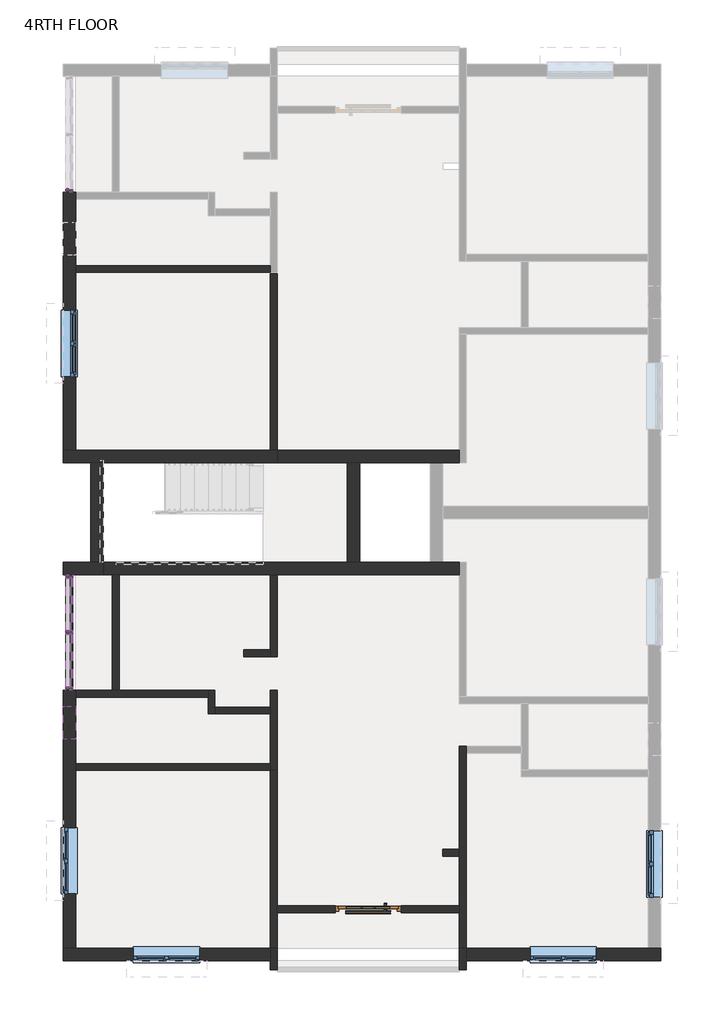
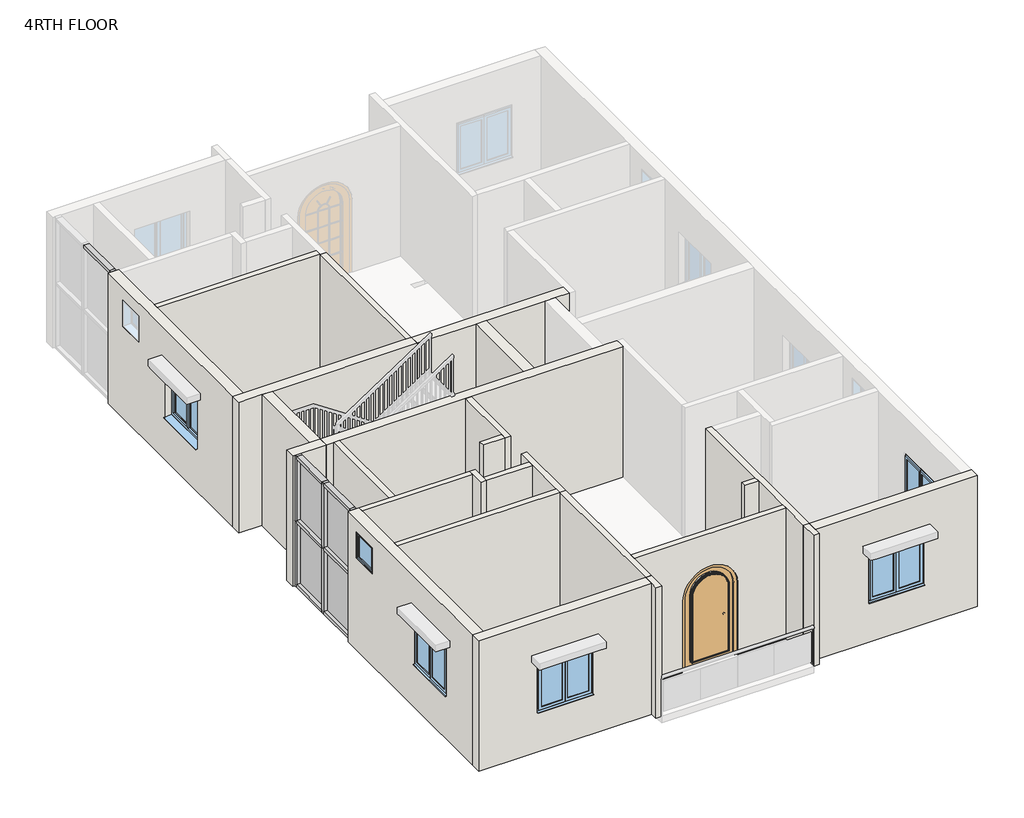
# One storey, part 1 of 4: 26 walls, 15 members, 6 windows, 4 plates, 1 door.
"""IFC4 building model written with IfcOpenShell, lengths in millimetres."""

from ifc_helpers import new_model, si_unit, point, frame, frame_2d, origin, place, context, project, spatial, polyline, circle_curve, trimmed, segment, composite_curve, outline, extrude, faceted_brep, transform, mapped, element, save
from components import door_arched_single_french_glass_wood_exterior_4_x_7_french_5c4dec95, member_801a2072, member_82905deb, member_88aa5c81, member_4491d118, system_panel_glazed_a8655be6, window_80340324, w2_windows_4_x_4_9dec5fc7

model = new_model("IFC4")

# Units and contexts
model_context = context("Model", 3, world=origin())
ifc_project = project(units=[si_unit("LENGTHUNIT", "METRE", prefix="MILLI")], contexts=[model_context])

# Site, building, storey
site = spatial("IfcSite", under=ifc_project)
building = spatial("IfcBuilding", under=site)
storey = spatial("IfcBuildingStorey", under=building, Name="4RTH FLOOR", Elevation=15240.0)

# Door
placement = place(None, origin())
door_arched_single_french_glass_wood_exterior_4_x_7_french_shape = door_arched_single_french_glass_wood_exterior_4_x_7_french_5c4dec95(model_context)
element("IfcDoor", 1, ObjectType="Door_Arched_Single_French_Glass_Wood_Exterior : 4' x 7' french door", at=placement, inside=storey, context=model_context, shape_type="MappedRepresentation", body=[
    mapped(door_arched_single_french_glass_wood_exterior_4_x_7_french_shape, transform((-817.6012202, -2286.2690997, 15240.0), x_axis=(-1.0, 0.0, 0.0), y_axis=(0.0, -1.0, 0.0), z_axis=(0.0, 0.0, 1.0))),
])

# Members
member_shape = member_801a2072(model_context)
element("IfcMember", 2, ObjectType="Rectangular Mullion : 2.5\" x 5\" rectangular", at=placement, inside=storey, context=model_context, shape_type="MappedRepresentation", body=[
    mapped(member_shape, transform((-6318.2887202, 10972.5309003, 18288.0), x_axis=(0.0, 0.0, 1.0), y_axis=(-1.0, 0.0, 0.0), z_axis=(0.0, -1.0, 0.0))),
])
element("IfcMember", 3, ObjectType="Rectangular Mullion : 2.5\" x 5\" rectangular", at=placement, inside=storey, context=model_context, shape_type="MappedRepresentation", body=[
    mapped(member_shape, transform((-6318.2887202, 1803.1309003, 18288.0), x_axis=(0.0, 0.0, 1.0), y_axis=(-1.0, 0.0, 0.0), z_axis=(0.0, -1.0, 0.0))),
])
element("IfcMember", 4, ObjectType="Rectangular Mullion : 2.5\" x 5\" rectangular", at=placement, inside=storey, context=model_context, shape_type="MappedRepresentation", body=[
    mapped(member_shape, transform((-6318.2887202, 2838.1809003, 18288.0), x_axis=(0.0, 0.0, 1.0), y_axis=(-1.0, 0.0, 0.0), z_axis=(0.0, -1.0, 0.0))),
])
element("IfcMember", 5, ObjectType="Rectangular Mullion : 2.5\" x 5\" rectangular", at=placement, inside=storey, context=model_context, shape_type="MappedRepresentation", body=[
    mapped(member_shape, transform((-6318.2887202, 3809.7309003, 15240.0), x_axis=(0.0, 0.0, -1.0), y_axis=(-1.0, 0.0, 0.0), z_axis=(0.0, 1.0, 0.0))),
])
element("IfcMember", 6, ObjectType="Rectangular Mullion : 2.5\" x 5\" rectangular", at=placement, inside=storey, context=model_context, shape_type="MappedRepresentation", body=[
    mapped(member_shape, transform((-6318.2887202, 2774.6809003, 15240.0), x_axis=(0.0, 0.0, -1.0), y_axis=(-1.0, 0.0, 0.0), z_axis=(0.0, 1.0, 0.0))),
])
member_2_shape = member_82905deb(model_context)
element("IfcMember", 7, ObjectType="Rectangular Mullion : 2.5\" x 5\" rectangular", at=placement, inside=storey, context=model_context, shape_type="MappedRepresentation", body=[
    mapped(member_2_shape, transform((-6318.2887202, 2806.4309003, 15240.0), x_axis=(0.0, -1.0, 0.0), y_axis=(-1.0, 0.0, 0.0), z_axis=(0.0, 0.0, -1.0))),
])
member_3_shape = member_88aa5c81(model_context)
element("IfcMember", 8, ObjectType="Rectangular Mullion : 2.5\" x 5\" rectangular", at=placement, inside=storey, context=model_context, shape_type="MappedRepresentation", body=[
    mapped(member_3_shape, transform((-6318.2887202, 2838.1809003, 16764.0), x_axis=(0.0, 0.0, 1.0), y_axis=(-1.0, 0.0, 0.0), z_axis=(0.0, -1.0, 0.0))),
])
element("IfcMember", 9, ObjectType="Rectangular Mullion : 2.5\" x 5\" rectangular", at=placement, inside=storey, context=model_context, shape_type="MappedRepresentation", body=[
    mapped(member_3_shape, transform((-6318.2887202, 1803.1309003, 16764.0), x_axis=(0.0, 0.0, 1.0), y_axis=(-1.0, 0.0, 0.0), z_axis=(0.0, -1.0, 0.0))),
])
element("IfcMember", 10, ObjectType="Rectangular Mullion : 2.5\" x 5\" rectangular", at=placement, inside=storey, context=model_context, shape_type="MappedRepresentation", body=[
    mapped(member_2_shape, transform((-6318.2887202, 2806.4309003, 16764.0), x_axis=(0.0, -1.0, 0.0), y_axis=(-1.0, 0.0, 0.0), z_axis=(0.0, 0.0, -1.0))),
])
member_4_shape = member_4491d118(model_context)
element("IfcMember", 11, ObjectType="Rectangular Mullion : 2.5\" x 5\" rectangular", at=placement, inside=storey, context=model_context, shape_type="MappedRepresentation", body=[
    mapped(member_4_shape, transform((-6318.2887202, 10909.0309003, 15240.0), x_axis=(0.0, -1.0, 0.0), y_axis=(-1.0, 0.0, 0.0), z_axis=(0.0, 0.0, -1.0))),
])
element("IfcMember", 12, ObjectType="Rectangular Mullion : 2.5\" x 5\" rectangular", at=placement, inside=storey, context=model_context, shape_type="MappedRepresentation", body=[
    mapped(member_4_shape, transform((-6318.2887202, 1739.6309003, 15240.0), x_axis=(0.0, -1.0, 0.0), y_axis=(-1.0, 0.0, 0.0), z_axis=(0.0, 0.0, -1.0))),
])
element("IfcMember", 13, ObjectType="Rectangular Mullion : 2.5\" x 5\" rectangular", at=placement, inside=storey, context=model_context, shape_type="MappedRepresentation", body=[
    mapped(member_4_shape, transform((-6318.2887202, 3873.2309003, 18288.0), x_axis=(0.0, 1.0, 0.0), y_axis=(-1.0, 0.0, 0.0), z_axis=(0.0, 0.0, 1.0))),
])
element("IfcMember", 14, ObjectType="Rectangular Mullion : 2.5\" x 5\" rectangular", at=placement, inside=storey, context=model_context, shape_type="MappedRepresentation", body=[
    mapped(member_4_shape, transform((-6318.2887202, 10909.0309003, 16764.0), x_axis=(0.0, -1.0, 0.0), y_axis=(-1.0, 0.0, 0.0), z_axis=(0.0, 0.0, -1.0))),
])
element("IfcMember", 15, ObjectType="Rectangular Mullion : 2.5\" x 5\" rectangular", at=placement, inside=storey, context=model_context, shape_type="MappedRepresentation", body=[
    mapped(member_4_shape, transform((-6318.2887202, 1739.6309003, 16764.0), x_axis=(0.0, -1.0, 0.0), y_axis=(-1.0, 0.0, 0.0), z_axis=(0.0, 0.0, -1.0))),
])
element("IfcMember", 16, ObjectType="Rectangular Mullion : 2.5\" x 5\" rectangular", at=placement, inside=storey, context=model_context, shape_type="MappedRepresentation", body=[
    mapped(member_4_shape, transform((-6318.2887202, 3873.2309003, 16764.0), x_axis=(0.0, 1.0, 0.0), y_axis=(-1.0, 0.0, 0.0), z_axis=(0.0, 0.0, 1.0))),
])

# Plates
system_panel_glazed_shape = system_panel_glazed_a8655be6(model_context)
element("IfcPlate", 17, ObjectType="System Panel : Glazed", at=placement, inside=storey, context=model_context, shape_type="MappedRepresentation", body=[
    mapped(system_panel_glazed_shape, transform((-6318.2887202, 3323.9559003, 15303.5), x_axis=(0.0, -1.0, 0.0), y_axis=(1.0, 0.0, 0.0), z_axis=(0.0, 0.0, 1.0))),
])
element("IfcPlate", 18, ObjectType="System Panel : Glazed", at=placement, inside=storey, context=model_context, shape_type="MappedRepresentation", body=[
    mapped(system_panel_glazed_shape, transform((-6318.2887202, 2288.9059003, 15303.5), x_axis=(0.0, -1.0, 0.0), y_axis=(1.0, 0.0, 0.0), z_axis=(0.0, 0.0, 1.0))),
])
element("IfcPlate", 19, ObjectType="System Panel : Glazed", at=placement, inside=storey, context=model_context, shape_type="MappedRepresentation", body=[
    mapped(system_panel_glazed_shape, transform((-6318.2887202, 3323.9559003, 16795.75), x_axis=(0.0, -1.0, 0.0), y_axis=(1.0, 0.0, 0.0), z_axis=(0.0, 0.0, 1.0))),
])
element("IfcPlate", 20, ObjectType="System Panel : Glazed", at=placement, inside=storey, context=model_context, shape_type="MappedRepresentation", body=[
    mapped(system_panel_glazed_shape, transform((-6318.2887202, 2288.9059003, 16795.75), x_axis=(0.0, -1.0, 0.0), y_axis=(1.0, 0.0, 0.0), z_axis=(0.0, 0.0, 1.0))),
])

# Walls
element("IfcWall", 21, ObjectType="OUTER WALL 9\"", at=placement, inside=storey, context=model_context, shape_type="Brep", body=[
    faceted_brep([(-6432.5887202, -3238.7690997, 15240.0), (-2621.0012202, -3238.7690997, 15240.0), (-2621.0012202, -3238.7690997, 18288.0), (-6432.5887202, -3238.7690997, 18288.0), (-5137.1887202, -3238.7690997, 16154.4), (-5137.1887202, -3238.7690997, 17373.6), (-3917.9887202, -3238.7690997, 17373.6), (-3917.9887202, -3238.7690997, 16154.4), (-6432.5887202, -3010.1690997, 15240.0), (-6432.5887202, -3010.1690997, 18288.0), (-6203.9887202, -3010.1690997, 18288.0), (-2621.0012202, -3010.1690997, 18288.0), (-2621.0012202, -3010.1690997, 15240.0), (-6203.9887202, -3010.1690997, 15240.0), (-5137.1887202, -3010.1690997, 16154.4), (-3917.9887202, -3010.1690997, 16154.4), (-3917.9887202, -3010.1690997, 17373.6), (-5137.1887202, -3010.1690997, 17373.6)], [[[0, 1, 2, 3], [4, 5, 6, 7]], [[8, 9, 10, 11, 12, 13], [14, 15, 16, 17]], [[1, 0, 8, 13, 12]], [[3, 2, 11, 10, 9]], [[0, 3, 9, 8]], [[2, 1, 12, 11]], [[5, 4, 14, 17]], [[6, 5, 17, 16]], [[7, 6, 16, 15]], [[4, 7, 15, 14]]]),
])
element("IfcWall", 22, ObjectType="OUTER WALL 9\"", at=placement, inside=storey, context=model_context, shape_type="Brep", body=[
    faceted_brep([(-6203.9887202, -3010.1690997, 18288.0), (-6203.9887202, -3010.1690997, 15240.0), (-6203.9887202, 266.4309003, 15240.0), (-6203.9887202, 393.4309003, 15240.0), (-6203.9887202, 1612.6309003, 15240.0), (-6203.9887202, 1739.6309003, 15240.0), (-6203.9887202, 1739.6309003, 18288.0), (-6203.9887202, 1612.6309003, 18288.0), (-6203.9887202, 393.4309003, 18288.0), (-6203.9887202, 266.4309003, 18288.0), (-6203.9887202, -787.6690997, 16240.0), (-6203.9887202, -2006.8690997, 16240.0), (-6203.9887202, -2006.8690997, 17459.2), (-6203.9887202, -787.6690997, 17459.2), (-6203.9887202, 1447.5309003, 17983.2), (-6203.9887202, 1447.5309003, 17373.6), (-6203.9887202, 837.9309003, 17373.6), (-6203.9887202, 837.9309003, 17983.2), (-6432.5887202, -3010.1690997, 15240.0), (-6432.5887202, -3010.1690997, 18288.0), (-6432.5887202, 1739.6309003, 18288.0), (-6432.5887202, 1739.6309003, 15240.0), (-6432.5887202, -787.6690997, 16240.0), (-6432.5887202, -787.6690997, 17459.2), (-6432.5887202, -2006.8690997, 17459.2), (-6432.5887202, -2006.8690997, 16240.0), (-6432.5887202, 1447.5309003, 17983.2), (-6432.5887202, 837.9309003, 17983.2), (-6432.5887202, 837.9309003, 17373.6), (-6432.5887202, 1447.5309003, 17373.6)], [[[0, 1, 2, 3, 4, 5, 6, 7, 8, 9], [10, 11, 12, 13], [14, 15, 16, 17]], [[18, 19, 20, 21], [22, 23, 24, 25], [26, 27, 28, 29]], [[1, 18, 21, 5, 4, 3, 2]], [[19, 0, 9, 8, 7, 6, 20]], [[1, 0, 19, 18]], [[6, 5, 21, 20]], [[23, 22, 10, 13]], [[24, 23, 13, 12]], [[25, 24, 12, 11]], [[22, 25, 11, 10]], [[15, 14, 26, 29]], [[16, 15, 29, 28]], [[17, 16, 28, 27]], [[14, 17, 27, 26]]]),
])
element("IfcWall", 23, ObjectType="OUTER WALL 9\"", at=placement, inside=storey, context=model_context, shape_type="Brep", body=[
    faceted_brep([(4567.1987798, -3010.1690997, 15240.0), (4338.5987798, -3010.1690997, 15240.0), (985.7987798, -3010.1690997, 15240.0), (985.7987798, -3010.1690997, 18288.0), (4338.5987798, -3010.1690997, 18288.0), (4567.1987798, -3010.1690997, 18288.0), (2166.8987798, -3010.1690997, 16154.4), (3386.0987798, -3010.1690997, 16154.4), (3386.0987798, -3010.1690997, 17373.6), (2166.8987798, -3010.1690997, 17373.6), (4567.1987798, -3238.7690997, 15240.0), (4567.1987798, -3238.7690997, 18288.0), (985.7987798, -3238.7690997, 18288.0), (985.7987798, -3238.7690997, 15240.0), (2166.8987798, -3238.7690997, 16154.4), (2166.8987798, -3238.7690997, 17373.6), (3386.0987798, -3238.7690997, 17373.6), (3386.0987798, -3238.7690997, 16154.4)], [[[0, 1, 2, 3, 4, 5], [6, 7, 8, 9]], [[10, 11, 12, 13], [14, 15, 16, 17]], [[2, 1, 0, 10, 13]], [[5, 4, 3, 12, 11]], [[0, 5, 11, 10]], [[15, 14, 6, 9]], [[16, 15, 9, 8]], [[17, 16, 8, 7]], [[14, 17, 7, 6]], [[3, 2, 13, 12]]]),
])
element("IfcWall", 24, ObjectType="OUTER WALL 9\"", at=placement, inside=storey, context=model_context, shape_type="SweptSolid", body=[
    extrude(outline(polyline([(6159.2309003, 15240.0), (6159.2309003, 18288.0), (10909.0309003, 18288.0), (10909.0309003, 15240.0), (6159.2309003, 15240.0)]), holes=[polyline([(7518.1309003, 16240.0), (8737.3309003, 16240.0), (8737.3309003, 17459.2), (7518.1309003, 17459.2), (7518.1309003, 16240.0)]), polyline([(9753.3309003, 17983.2), (9753.3309003, 17373.6), (10362.9309003, 17373.6), (10362.9309003, 17983.2), (9753.3309003, 17983.2)])]), frame((-6432.5887202, 0.0, 0.0), z_axis=(1.0, 0.0, 0.0), x_axis=(0.0, 1.0, 0.0)), (0.0, 0.0, 1.0), 228.6),
])
element("IfcWall", 25, ObjectType="OUTER WALL 9\"", at=placement, inside=storey, context=model_context, shape_type="Brep", body=[
    faceted_brep([(-6432.5887202, 5930.6309003, 15240.0), (-5923.0012202, 5930.6309003, 15240.0), (-5694.4012202, 5930.6309003, 15240.0), (-2494.0012202, 5930.6309003, 15240.0), (-2494.0012202, 5930.6309003, 18288.0), (-5694.4012202, 5930.6309003, 18288.0), (-5923.0012202, 5930.6309003, 18288.0), (-6432.5887202, 5930.6309003, 18288.0), (-6432.5887202, 6159.2309003, 15240.0), (-6432.5887202, 6159.2309003, 18288.0), (-6203.9887202, 6159.2309003, 18288.0), (-2621.0012202, 6159.2309003, 18288.0), (-2494.0012202, 6159.2309003, 18288.0), (-2494.0012202, 6159.2309003, 15240.0), (-2621.0012202, 6159.2309003, 15240.0), (-6203.9887202, 6159.2309003, 15240.0)], [[[0, 1, 2, 3, 4, 5, 6, 7]], [[8, 9, 10, 11, 12, 13, 14, 15]], [[3, 2, 1, 0, 8, 15, 14, 13]], [[7, 6, 5, 4, 12, 11, 10, 9]], [[0, 7, 9, 8]], [[4, 3, 13, 12]]]),
])
element("IfcWall", 26, ObjectType="OUTER WALL 9\"", at=placement, inside=storey, context=model_context, shape_type="SweptSolid", body=[
    extrude(outline(polyline([(-5923.0012202, 4101.8309003), (-5923.0012202, 5930.6309003), (-5694.4012202, 5930.6309003), (-5694.4012202, 4101.8309003), (-5923.0012202, 4101.8309003)])), frame((0.0, 0.0, 15240.0), z_axis=(0.0, 0.0, 1.0), x_axis=(1.0, 0.0, 0.0)), (0.0, 0.0, 1.0), 3048.0),
])
element("IfcWall", 27, ObjectType="OUTER WALL 9\"", at=placement, inside=storey, context=model_context, shape_type="Brep", body=[
    faceted_brep([(-5694.4012202, 4101.8309003, 15240.0), (-5923.0012202, 4101.8309003, 15240.0), (-6432.5887202, 4101.8309003, 15240.0), (-6432.5887202, 4101.8309003, 18288.0), (-5923.0012202, 4101.8309003, 18288.0), (-5694.4012202, 4101.8309003, 18288.0), (-5694.4012202, 3873.2309003, 15240.0), (-5694.4012202, 3873.2309003, 18288.0), (-6432.5887202, 3873.2309003, 18288.0), (-6432.5887202, 3873.2309003, 15240.0)], [[[0, 1, 2, 3, 4, 5]], [[6, 7, 8, 9]], [[2, 1, 0, 6, 9]], [[5, 4, 3, 8, 7]], [[0, 5, 7, 6]], [[3, 2, 9, 8]]]),
])
element("IfcWall", 28, ObjectType="OUTER WALL 9\"", at=placement, inside=storey, context=model_context, shape_type="Brep", body=[
    faceted_brep([(-5694.4012202, 3873.2309003, 15240.0), (-5529.3012202, 3873.2309003, 15240.0), (-5402.3012202, 3873.2309003, 15240.0), (-2621.0012202, 3873.2309003, 15240.0), (-2494.0012202, 3873.2309003, 15240.0), (858.7987798, 3873.2309003, 15240.0), (858.7987798, 3873.2309003, 18288.0), (-2494.0012202, 3873.2309003, 18288.0), (-2621.0012202, 3873.2309003, 18288.0), (-5402.3012202, 3873.2309003, 18288.0), (-5529.3012202, 3873.2309003, 18288.0), (-5694.4012202, 3873.2309003, 18288.0), (-5694.4012202, 4101.8309003, 15240.0), (-5694.4012202, 4101.8309003, 18288.0), (-1198.6012202, 4101.8309003, 18288.0), (-970.0012202, 4101.8309003, 18288.0), (325.3987798, 4101.8309003, 18288.0), (553.9987798, 4101.8309003, 18288.0), (858.7987798, 4101.8309003, 18288.0), (858.7987798, 4101.8309003, 15240.0), (553.9987798, 4101.8309003, 15240.0), (325.3987798, 4101.8309003, 15240.0), (-970.0012202, 4101.8309003, 15240.0), (-1198.6012202, 4101.8309003, 15240.0)], [[[0, 1, 2, 3, 4, 5, 6, 7, 8, 9, 10, 11]], [[12, 13, 14, 15, 16, 17, 18, 19, 20, 21, 22, 23]], [[5, 4, 3, 2, 1, 0, 12, 23, 22, 21, 20, 19]], [[11, 10, 9, 8, 7, 6, 18, 17, 16, 15, 14, 13]], [[0, 11, 13, 12]], [[6, 5, 19, 18]]]),
])
element("IfcWall", 29, ObjectType="OUTER WALL 9\"", at=placement, inside=storey, context=model_context, shape_type="Brep", body=[
    faceted_brep([(858.7987798, 6159.2309003, 15240.0), (-2494.0012202, 6159.2309003, 15240.0), (-2494.0012202, 6159.2309003, 18288.0), (858.7987798, 6159.2309003, 18288.0), (858.7987798, 5930.6309003, 15240.0), (858.7987798, 5930.6309003, 18288.0), (553.9987798, 5930.6309003, 18288.0), (325.3987798, 5930.6309003, 18288.0), (-970.0012202, 5930.6309003, 18288.0), (-1198.6012202, 5930.6309003, 18288.0), (-2494.0012202, 5930.6309003, 18288.0), (-2494.0012202, 5930.6309003, 15240.0), (-1198.6012202, 5930.6309003, 15240.0), (-970.0012202, 5930.6309003, 15240.0), (325.3987798, 5930.6309003, 15240.0), (553.9987798, 5930.6309003, 15240.0)], [[[0, 1, 2, 3]], [[4, 5, 6, 7, 8, 9, 10, 11, 12, 13, 14, 15]], [[1, 0, 4, 15, 14, 13, 12, 11]], [[3, 2, 10, 9, 8, 7, 6, 5]], [[2, 1, 11, 10]], [[0, 3, 5, 4]]]),
])
element("IfcWall", 30, ObjectType="OUTER WALL 9\"", at=placement, inside=storey, context=model_context, shape_type="SweptSolid", body=[
    extrude(outline(polyline([(-1198.6012202, 4101.8309003), (-1198.6012202, 5930.6309003), (-970.0012202, 5930.6309003), (-970.0012202, 4101.8309003), (-1198.6012202, 4101.8309003)])), frame((0.0, 0.0, 15240.0), z_axis=(0.0, 0.0, 1.0), x_axis=(1.0, 0.0, 0.0)), (0.0, 0.0, 1.0), 3048.0),
])
element("IfcWall", 31, ObjectType="inner wall 5\"", at=placement, inside=storey, context=model_context, shape_type="SweptSolid", body=[
    extrude(outline(polyline([(-6202.4012202, 9562.8309003), (-2621.0012202, 9562.8309003), (-2621.0012202, 9435.8309003), (-6202.4012202, 9435.8309003), (-6202.4012202, 9562.8309003)])), frame((0.0, 0.0, 15240.0), z_axis=(0.0, 0.0, 1.0), x_axis=(1.0, 0.0, 0.0)), (0.0, 0.0, 1.0), 3048.0),
])
element("IfcWall", 32, ObjectType="inner wall 5\"", at=placement, inside=storey, context=model_context, shape_type="SweptSolid", body=[
    extrude(outline(polyline([(-5529.3012202, 1739.6309003), (-5529.3012202, 3873.2309003), (-5402.3012202, 3873.2309003), (-5402.3012202, 1739.6309003), (-5529.3012202, 1739.6309003)])), frame((0.0, 0.0, 15240.0), z_axis=(0.0, 0.0, 1.0), x_axis=(1.0, 0.0, 0.0)), (0.0, 0.0, 1.0), 3048.0),
])
element("IfcWall", 33, ObjectType="inner wall 5\"", at=placement, inside=storey, context=model_context, shape_type="Brep", body=[
    faceted_brep([(-2621.0012202, 3873.2309003, 15240.0), (-2621.0012202, 2488.9309003, 15240.0), (-2621.0012202, 2361.9309003, 15240.0), (-2621.0012202, 2361.9309003, 18288.0), (-2621.0012202, 2488.9309003, 18288.0), (-2621.0012202, 3873.2309003, 18288.0), (-2494.0012202, 3873.2309003, 15240.0), (-2494.0012202, 3873.2309003, 18288.0), (-2494.0012202, 2361.9309003, 18288.0), (-2494.0012202, 2361.9309003, 15240.0)], [[[0, 1, 2, 3, 4, 5]], [[6, 7, 8, 9]], [[2, 1, 0, 6, 9]], [[5, 4, 3, 8, 7]], [[0, 5, 7, 6]], [[3, 2, 9, 8]]]),
])
element("IfcWall", 34, ObjectType="inner wall 5\"", at=placement, inside=storey, context=model_context, shape_type="SweptSolid", body=[
    extrude(outline(polyline([(-3103.6012202, 2488.9309003), (-2621.0012202, 2488.9309003), (-2621.0012202, 2361.9309003), (-3103.6012202, 2361.9309003), (-3103.6012202, 2488.9309003)])), frame((0.0, 0.0, 15240.0), z_axis=(0.0, 0.0, 1.0), x_axis=(1.0, 0.0, 0.0)), (0.0, 0.0, 1.0), 3048.0),
])
element("IfcWall", 35, ObjectType="inner wall 5\"", at=placement, inside=storey, context=model_context, shape_type="Brep", body=[
    faceted_brep([(-6203.9887202, 1612.6309003, 15240.0), (-3764.0012202, 1612.6309003, 15240.0), (-3764.0012202, 1612.6309003, 18288.0), (-6203.9887202, 1612.6309003, 18288.0), (-6203.9887202, 1739.6309003, 15240.0), (-6203.9887202, 1739.6309003, 18288.0), (-5529.3012202, 1739.6309003, 18288.0), (-5402.3012202, 1739.6309003, 18288.0), (-3764.0012202, 1739.6309003, 18288.0), (-3764.0012202, 1739.6309003, 15240.0), (-5402.3012202, 1739.6309003, 15240.0), (-5529.3012202, 1739.6309003, 15240.0)], [[[0, 1, 2, 3]], [[4, 5, 6, 7, 8, 9, 10, 11]], [[1, 0, 4, 11, 10, 9]], [[3, 2, 8, 7, 6, 5]], [[0, 3, 5, 4]], [[2, 1, 9, 8]]]),
])
element("IfcWall", 36, ObjectType="inner wall 5\"", at=placement, inside=storey, context=model_context, shape_type="Brep", body=[
    faceted_brep([(-3764.0012202, 1739.6309003, 15240.0), (-3764.0012202, 1612.6309003, 15240.0), (-3764.0012202, 1307.8309003, 15240.0), (-3764.0012202, 1307.8309003, 18288.0), (-3764.0012202, 1612.6309003, 18288.0), (-3764.0012202, 1739.6309003, 18288.0), (-3637.0012202, 1739.6309003, 15240.0), (-3637.0012202, 1739.6309003, 18288.0), (-3637.0012202, 1434.8309003, 18288.0), (-3637.0012202, 1307.8309003, 18288.0), (-3637.0012202, 1307.8309003, 15240.0), (-3637.0012202, 1434.8309003, 15240.0)], [[[0, 1, 2, 3, 4, 5]], [[6, 7, 8, 9, 10, 11]], [[2, 1, 0, 6, 11, 10]], [[5, 4, 3, 9, 8, 7]], [[0, 5, 7, 6]], [[3, 2, 10, 9]]]),
])
element("IfcWall", 37, ObjectType="inner wall 5\"", at=placement, inside=storey, context=model_context, shape_type="SweptSolid", body=[
    extrude(outline(polyline([(-2621.0012202, 1307.8309003), (-3637.0012202, 1307.8309003), (-3637.0012202, 1434.8309003), (-2621.0012202, 1434.8309003), (-2621.0012202, 1307.8309003)])), frame((0.0, 0.0, 15240.0), z_axis=(0.0, 0.0, 1.0), x_axis=(1.0, 0.0, 0.0)), (0.0, 0.0, 1.0), 3048.0),
])
element("IfcWall", 38, ObjectType="inner wall 5\"", at=placement, inside=storey, context=model_context, shape_type="Brep", body=[
    faceted_brep([(-2621.0012202, 1739.6309003, 15240.0), (-2621.0012202, 1434.8309003, 15240.0), (-2621.0012202, 1307.8309003, 15240.0), (-2621.0012202, 393.4309003, 15240.0), (-2621.0012202, 266.4309003, 15240.0), (-2621.0012202, 266.4309003, 18288.0), (-2621.0012202, 393.4309003, 18288.0), (-2621.0012202, 1307.8309003, 18288.0), (-2621.0012202, 1434.8309003, 18288.0), (-2621.0012202, 1739.6309003, 18288.0), (-2494.0012202, 1739.6309003, 15240.0), (-2494.0012202, 1739.6309003, 18288.0), (-2494.0012202, 266.4309003, 18288.0), (-2494.0012202, 266.4309003, 15240.0)], [[[0, 1, 2, 3, 4, 5, 6, 7, 8, 9]], [[10, 11, 12, 13]], [[4, 3, 2, 1, 0, 10, 13]], [[9, 8, 7, 6, 5, 12, 11]], [[0, 9, 11, 10]], [[5, 4, 13, 12]]]),
])
element("IfcWall", 39, ObjectType="inner wall 5\"", at=placement, inside=storey, context=model_context, shape_type="SweptSolid", body=[
    extrude(outline(polyline([(-6203.9887202, 393.4309003), (-2621.0012202, 393.4309003), (-2621.0012202, 266.4309003), (-6203.9887202, 266.4309003), (-6203.9887202, 393.4309003)])), frame((0.0, 0.0, 15240.0), z_axis=(0.0, 0.0, 1.0), x_axis=(1.0, 0.0, 0.0)), (0.0, 0.0, 1.0), 3048.0),
])
element("IfcWall", 40, ObjectType="inner wall 5\"", at=placement, inside=storey, context=model_context, shape_type="Brep", body=[
    faceted_brep([(-2494.0012202, -3010.1690997, 15240.0), (-2494.0012202, -2349.7690997, 15240.0), (-2494.0012202, -2222.7690997, 15240.0), (-2494.0012202, 266.4309003, 15240.0), (-2494.0012202, 266.4309003, 18288.0), (-2494.0012202, -2222.7690997, 18288.0), (-2494.0012202, -2349.7690997, 18288.0), (-2494.0012202, -3010.1690997, 18288.0), (-2621.0012202, -3010.1690997, 15240.0), (-2621.0012202, -3010.1690997, 18288.0), (-2621.0012202, 266.4309003, 18288.0), (-2621.0012202, 266.4309003, 15240.0)], [[[0, 1, 2, 3, 4, 5, 6, 7]], [[8, 9, 10, 11]], [[3, 2, 1, 0, 8, 11]], [[7, 6, 5, 4, 10, 9]], [[4, 3, 11, 10]], [[0, 7, 9, 8]]]),
])
element("IfcWall", 41, ObjectType="inner wall 5\"", at=placement, inside=storey, context=model_context, shape_type="Brep", body=[
    faceted_brep([(985.7987798, -3010.1690997, 15240.0), (985.7987798, 583.9309003, 15240.0), (985.7987798, 710.9309003, 15240.0), (985.7987798, 710.9309003, 18288.0), (985.7987798, 583.9309003, 18288.0), (985.7987798, -3010.1690997, 18288.0), (858.7987798, -3010.1690997, 15240.0), (858.7987798, -3010.1690997, 18288.0), (858.7987798, -2349.7690997, 18288.0), (858.7987798, -2222.7690997, 18288.0), (858.7987798, -1308.3690997, 18288.0), (858.7987798, -1181.3690997, 18288.0), (858.7987798, 710.9309003, 18288.0), (858.7987798, 710.9309003, 15240.0), (858.7987798, -1181.3690997, 15240.0), (858.7987798, -1308.3690997, 15240.0), (858.7987798, -2222.7690997, 15240.0), (858.7987798, -2349.7690997, 15240.0)], [[[0, 1, 2, 3, 4, 5]], [[6, 7, 8, 9, 10, 11, 12, 13, 14, 15, 16, 17]], [[2, 1, 0, 6, 17, 16, 15, 14, 13]], [[5, 4, 3, 12, 11, 10, 9, 8, 7]], [[3, 2, 13, 12]], [[0, 5, 7, 6]]]),
])
element("IfcWall", 42, ObjectType="inner wall 5\"", at=placement, inside=storey, context=model_context, shape_type="Brep", body=[
    faceted_brep([(-2621.0012202, -3010.1690997, 15240.0), (-2621.0012202, -3238.7690997, 15240.0), (-2621.0012202, -3403.8690997, 15240.0), (-2621.0012202, -3403.8690997, 18288.0), (-2621.0012202, -3238.7690997, 18288.0), (-2621.0012202, -3010.1690997, 18288.0), (-2494.0012202, -3010.1690997, 15240.0), (-2494.0012202, -3010.1690997, 18288.0), (-2494.0012202, -3403.8690997, 18288.0), (-2494.0012202, -3403.8690997, 15240.0)], [[[0, 1, 2, 3, 4, 5]], [[6, 7, 8, 9]], [[2, 1, 0, 6, 9]], [[3, 2, 9, 8]], [[5, 4, 3, 8, 7]], [[0, 5, 7, 6]]]),
])
element("IfcWall", 43, ObjectType="inner wall 5\"", at=placement, inside=storey, context=model_context, shape_type="SweptSolid", body=[
    extrude(outline(composite_curve([segment(polyline([(15240.0, -2494.0012202), (15240.0, -1427.2012202), (16918.6, -1427.2012202)]), True, "CONTINUOUS"), segment(trimmed(circle_curve(frame_2d((16918.6, -817.6012202)), 609.6), [point((16918.6, -1427.2012202))], [point((16918.6, -208.0012202))], True, "CARTESIAN"), True, "CONTINUOUS"), segment(polyline([(16918.6, -208.0012202), (15240.0, -208.0012202), (15240.0, 858.7987798), (18288.0, 858.7987798), (18288.0, -2494.0012202), (15240.0, -2494.0012202)]), True, "CONTINUOUS")], self_intersect=False)), frame((0.0, -2349.7690997, 0.0), z_axis=(0.0, 1.0, 0.0), x_axis=(0.0, 0.0, 1.0)), (0.0, 0.0, 1.0), 127.0),
])
element("IfcWall", 44, ObjectType="inner wall 5\"", at=placement, inside=storey, context=model_context, shape_type="SweptSolid", body=[
    extrude(outline(polyline([(553.9987798, -1181.3690997), (858.7987798, -1181.3690997), (858.7987798, -1308.3690997), (553.9987798, -1308.3690997), (553.9987798, -1181.3690997)])), frame((0.0, 0.0, 15240.0), z_axis=(0.0, 0.0, 1.0), x_axis=(1.0, 0.0, 0.0)), (0.0, 0.0, 1.0), 3048.0),
])
element("IfcWall", 45, ObjectType="inner wall 5\"", at=placement, inside=storey, context=model_context, shape_type="SweptSolid", body=[
    extrude(outline(polyline([(-2621.0012202, 6159.2309003), (-2621.0012202, 9410.4309003), (-2494.0012202, 9410.4309003), (-2494.0012202, 6159.2309003), (-2621.0012202, 6159.2309003)])), frame((0.0, 0.0, 15240.0), z_axis=(0.0, 0.0, 1.0), x_axis=(1.0, 0.0, 0.0)), (0.0, 0.0, 1.0), 3048.0),
])
element("IfcWall", 46, ObjectType="inner wall 5\"", at=placement, inside=storey, context=model_context, shape_type="Brep", body=[
    faceted_brep([(858.7987798, -3010.1690997, 15240.0), (858.7987798, -3403.8690997, 15240.0), (858.7987798, -3403.8690997, 18288.0), (858.7987798, -3010.1690997, 18288.0), (985.7987798, -3010.1690997, 15240.0), (985.7987798, -3010.1690997, 18288.0), (985.7987798, -3238.7690997, 18288.0), (985.7987798, -3403.8690997, 18288.0), (985.7987798, -3403.8690997, 15240.0), (985.7987798, -3238.7690997, 15240.0)], [[[0, 1, 2, 3]], [[4, 5, 6, 7, 8, 9]], [[1, 0, 4, 9, 8]], [[2, 1, 8, 7]], [[3, 2, 7, 6, 5]], [[0, 3, 5, 4]]]),
])

# Windows
window_shape = window_80340324(model_context)
element("IfcWindow", 47, ObjectType="Fixed : 24\" x 24\"", at=placement, inside=storey, context=model_context, shape_type="MappedRepresentation", body=[
    mapped(window_shape, transform((-6318.2887202, 1180.8309003, 16459.2), x_axis=(0.0, 1.0, 0.0), y_axis=(-1.0, 0.0, 0.0), z_axis=(0.0, 0.0, 1.0))),
])
w2_windows_4_x_4_shape = w2_windows_4_x_4_9dec5fc7(model_context)
element("IfcWindow", 48, ObjectType="w2 : windows 4' x 4'", at=placement, inside=storey, context=model_context, shape_type="MappedRepresentation", body=[
    mapped(w2_windows_4_x_4_shape, transform((-4527.5887202, -3124.4690997, 15154.4), x_axis=(1.0, 0.0, 0.0), y_axis=(0.0, 1.0, 0.0), z_axis=(0.0, 0.0, 1.0))),
])
element("IfcWindow", 49, ObjectType="w2 : windows 4' x 4'", at=placement, inside=storey, context=model_context, shape_type="MappedRepresentation", body=[
    mapped(w2_windows_4_x_4_shape, transform((2776.4987798, -3124.4690997, 15154.4), x_axis=(1.0, 0.0, 0.0), y_axis=(0.0, 1.0, 0.0), z_axis=(0.0, 0.0, 1.0))),
])
element("IfcWindow", 50, ObjectType="w2 : windows 4' x 4'", at=placement, inside=storey, context=model_context, shape_type="MappedRepresentation", body=[
    mapped(w2_windows_4_x_4_shape, transform((-6318.2887202, 8127.7309003, 15240.0), x_axis=(0.0, 1.0, 0.0), y_axis=(-1.0, 0.0, 0.0), z_axis=(0.0, 0.0, 1.0))),
])
element("IfcWindow", 51, ObjectType="w2 : windows 4' x 4'", at=placement, inside=storey, context=model_context, shape_type="MappedRepresentation", body=[
    mapped(w2_windows_4_x_4_shape, transform((4452.8987798, -1454.4190997, 15240.0), x_axis=(0.0, -1.0, 0.0), y_axis=(1.0, 0.0, 0.0), z_axis=(0.0, 0.0, 1.0))),
])
element("IfcWindow", 52, ObjectType="w2 : windows 4' x 4'", at=placement, inside=storey, context=model_context, shape_type="MappedRepresentation", body=[
    mapped(w2_windows_4_x_4_shape, transform((-6318.2887202, -1397.2690997, 15240.0), x_axis=(0.0, -1.0, 0.0), y_axis=(1.0, 0.0, 0.0), z_axis=(0.0, 0.0, 1.0))),
])

save(model, "model.ifc")

# Revit data of these elements
# Type "Door_Arched_Single_French_Glass_Wood_Exterior : 4' x 7' french door"
#   Type Mark = "17"
#   Type Comments = "External Single"
#   Operation = "SingleSwingRight"
#   Keynote = "L20"
#   Analytic Construction = "<None>"
#   Wrap Layers (Int) from Ext = 0' - 6.98819"
#   Wrap Layers (Ext) from Ext = 0' - 4.03543"
#   Thickness = 0' - 1.73228"
#   Stile Shutting = 0' - 5.90551"
#   Stile - Top Rail = 0' - 5.90551"
#   Stile - Hanging = 0' - 5.90551"
#   Stile - Bottom Rail = 0' - 6.88976"
#   Rough Width = 4' - 0"
#   Rough Height = 7' - 0"
#   O/A Frame Width = 0' - 2.51969"
#   Handle Z Distance = 3' - 5.33858"
#   Glazing Thickness = 0' - 0.94488"
#   Glazing Bar Thickness = 0' - 0.7874"
#   FrameWidth = 0' - 1.65354"
#   FrameOffset - External = 0' - 0.98425"
#   FrameDepth = 0' - 3.50394"
#   Door Panel Width = 3' - 7.94488"
#   Handle X Distance = 0' - 2.95276"
#   Height = 7' - 0"
#   Structural Tolerance = 0' - 0.25591"
#   Tolerance = 0' - 0.11811"
#   Undercut = 0' - 0.15748"
#   Width = 4' - 0"
#   Door Panel Thickness = 0' - 1.73228"
#   Door Panel Height = 6' - 9.81496"
#   Cavity Closer Width = 0' - 1.9685"
#   Cavity Closer Offset from Ext = 0' - 4.03543"
#   Cavity Closer Depth = 0' - 3.34646"
#   Vis - Ironmongery = yes
#   Vis - Cavity Closers = yes
#   Define Thermal Properties by = 1
#   Material Glass = Door - Glazing
#   Handle Style = element 430241
#   Material Door = Door - Panel
#   Material Frame = BROWN
#   Material Ironmongery = Door - Handle
#   Function = (empty or 0)
#   Wall Closure = (empty or 0)
#   Assembly Code = ""
# Type "Rectangular Mullion : 2.5\" x 5\" rectangular"
#   built-in parameter 1007304 = 0.416667 (stored number, unit not read)
#   built-in parameter 1007301 = 0.104167 (stored number, unit not read)
#   built-in parameter 1007300 = 0.104167 (stored number, unit not read)
# Type "System Panel : Glazed"
#   Construction Type Id = "GSP4R"
#   Analytic Construction = "1/8 in Pilkington single glazing"
#   Visual Light Transmittance = 0.9
#   Solar Heat Gain Coefficient = 0.86
#   Heat Transfer Coefficient (U) = 1.18115 BTU/(h·ft²·°F)
#   Define Thermal Properties by = 1
# Type "OUTER WALL 9\""
#   Assembly Code = "B2010"
#   Layers, outside or top first: 0' - 9" "ROSE COLOUR" (function 1)
# Type "inner wall 5\""
#   Assembly Code = "B2010"
#   Layers, outside or top first: 0' - 5" "ROSE COLOUR" (function 1)
# Type "Fixed : 24\" x 24\""
#   Type Mark = "3"
#   Construction Type Id = "GSP4R"
#   Assembly Code = "B2020100"
#   Analytic Construction = "1/8 in Pilkington single glazing"
#   Visual Light Transmittance = 0.9
#   Solar Heat Gain Coefficient = 0.78
#   Heat Transfer Coefficient (U) = 0.6496 BTU/(h·ft²·°F)
#   Height = 2' - 0"
#   Default Sill Height = 3' - 0"
#   Width = 2' - 0"
#   Window Inset = 0' - 0 3/4"
#   Define Thermal Properties by = 1
#   Define Thermal Properties by = 1
#   Glass Pane Material = Glass
#   Sash Material = Sash
#   Wall Closure = (empty or 0)
# Type "w2 : windows 4' x 4'"
#   Type Mark = "31"
#   Operation = "DoublePanelVertical"
#   Keynote = "16.05.01"
#   Analytic Construction = "<None>"
#   Rough Width = 4' - 0"
#   Rough Height = 4' - 0"
#   Rahmentiefe = 0' - 2.3622"
#   Rahmenhöhe unten = 0' - 3.14961"
#   Rahmehöhe oben = 0' - 3.14961"
#   Rahmenbreite = 0' - 2.3622"
#   Heat Transfer Coefficient (U) = 2.81836 BTU/(h·ft²·°F)
#   Height = 4' - 0"
#   Flügeltiefe = 0' - 2.3622"
#   Flügelbreite = 0' - 2.3622"
#   Einbautiefe (von außen) [instance default] = 0' - 5.51181"
#   Width = 4' - 0"
#   Kippflügel [instance default] = yes
#   Drehflügel im Grundriß darstellen [instance default] = no
#   Drehflügel [instance default] = yes
#   Define Thermal Properties by = 1
#   Rahmen [instance default] = none
#   Glas [instance default] = blue glass
#   Flügel [instance default] = WINDOW COLOUR WHITE
#   Fensterbank aussen [instance default] = WINDOW COLOUR WHITE
#   Fensterbank innen [instance default] = WINDOW COLOUR WHITE
#   Visual Light Transmittance = 0
#   Thermal Resistance (R) = 0
#   Solar Heat Gain Coefficient = 0
#   Wall Closure = (empty or 0)
# Element 1 (IfcDoor, "Door_Arched_Single_French_Glass_Wood_Exterior : 4' x 7' french door")
#   Phase Created = New Construction
#   Materials on its faces: "Door - Panel", "Door - Handle", "BROWN", "Door - Glazing"
# Elements 2, 3, 4, 5, 6, 7, 8, 9, 10, 11, 12, 13, 14, 15, 16 (IfcMember, "Rectangular Mullion : 2.5\" x 5\" rectangular")
#   Phase Created = New Construction
#   Materials on its faces: "Aluminum"
# Elements 17, 18, 19, 20 (IfcPlate, "System Panel : Glazed")
#   Phase Created = New Construction
#   Materials on its faces: "Glass"
# Elements 21, 22, 23, 24, 25, 26, 27, 28, 29, 30 (IfcWall, "OUTER WALL 9\"")
#   Top Offset = 0' - 0"
#   Base Offset = 0' - 0"
#   wall height = 10' - 0"
#   Phase Created = New Construction
#   Base Constraint = 4RTH FLOOR
#   Top Constraint = 5th floor
#   Materials on its faces: "ROSE COLOUR"
# Elements 31, 32, 33, 34, 35, 36, 37, 38, 39, 40, 41, 42, 43, 44, 45, 46 (IfcWall, "inner wall 5\"")
#   Top Offset = 0' - 0"
#   Base Offset = 0' - 0"
#   wall height = 10' - 0"
#   Phase Created = New Construction
#   Base Constraint = 4RTH FLOOR
#   Top Constraint = 5th floor
#   Materials on its faces: "ROSE COLOUR"
# Element 47 (IfcWindow, "Fixed : 24\" x 24\"")
#   Mark = "77"
#   Phase Created = New Construction
#   Materials on its faces: "Sash", "Glass"
# Element 48 (IfcWindow, "w2 : windows 4' x 4'")
#   Mark = "69"
#   Phase Created = New Construction
#   Materials on its faces: "WINDOW COLOUR WHITE", "blue glass"
# Element 49 (IfcWindow, "w2 : windows 4' x 4'")
#   Mark = "70"
#   Phase Created = New Construction
#   Materials on its faces: "WINDOW COLOUR WHITE", "blue glass"
# Element 50 (IfcWindow, "w2 : windows 4' x 4'")
#   Mark = "73"
#   Einbautiefe (von außen) = 0' - 5.51181"
#   Kippflügel = yes
#   Drehflügel im Grundriß darstellen = no
#   Drehflügel = yes
#   Rahmen = none
#   Glas = blue glass
#   Flügel = WINDOW COLOUR WHITE
#   Fensterbank innen = WINDOW COLOUR WHITE
#   Fensterbank aussen = WINDOW COLOUR WHITE
#   Phase Created = New Construction
#   Materials on its faces: "WINDOW COLOUR WHITE", "blue glass"
# Element 51 (IfcWindow, "w2 : windows 4' x 4'")
#   Mark = "74"
#   Einbautiefe (von außen) = 0' - 5.51181"
#   Kippflügel = yes
#   Drehflügel im Grundriß darstellen = no
#   Drehflügel = yes
#   Rahmen = none
#   Glas = blue glass
#   Flügel = WINDOW COLOUR WHITE
#   Fensterbank innen = WINDOW COLOUR WHITE
#   Fensterbank aussen = WINDOW COLOUR WHITE
#   Phase Created = New Construction
#   Materials on its faces: "WINDOW COLOUR WHITE", "blue glass"
# Element 52 (IfcWindow, "w2 : windows 4' x 4'")
#   Mark = "75"
#   Einbautiefe (von außen) = 0' - 5.51181"
#   Kippflügel = yes
#   Drehflügel im Grundriß darstellen = no
#   Drehflügel = yes
#   Rahmen = none
#   Glas = blue glass
#   Flügel = WINDOW COLOUR WHITE
#   Fensterbank innen = WINDOW COLOUR WHITE
#   Fensterbank aussen = WINDOW COLOUR WHITE
#   Phase Created = New Construction
#   Materials on its faces: "WINDOW COLOUR WHITE", "blue glass"
# Materials
#   "Door - Glazing": colour RGB 218 227 224, transparency 0.85
#   "Door - Panel": class "Wood", colour RGB 210 159 95, transparency 0, Cost = 0
#   "BROWN": class "Generic", colour RGB 120 120 120, transparency 0, Cost = 0
#   "Door - Handle": colour RGB 0 0 0, transparency 0, Keynote = "P21"
#   "ROSE COLOUR": class "Generic", colour RGB 120 120 120, transparency 0, Cost = 0
#   "Glass": class "Glass", colour RGB 0 128 192, transparency 0.75, Description = "Soda Lime Glass", Cost = 0
#   "Sash": class "Wood", colour RGB 224 178 126, transparency 0, Cost = 0
#   "blue glass": class "System", colour RGB 0 0 255, transparency 0.75, Cost = 0
#   "WINDOW COLOUR WHITE": class "Generic", colour RGB 120 120 120, transparency 0, Cost = 0
#   "Aluminum": class "Metal", colour RGB 247 247 247, transparency 0, Description = "Aluminum 6061", Cost = 0
